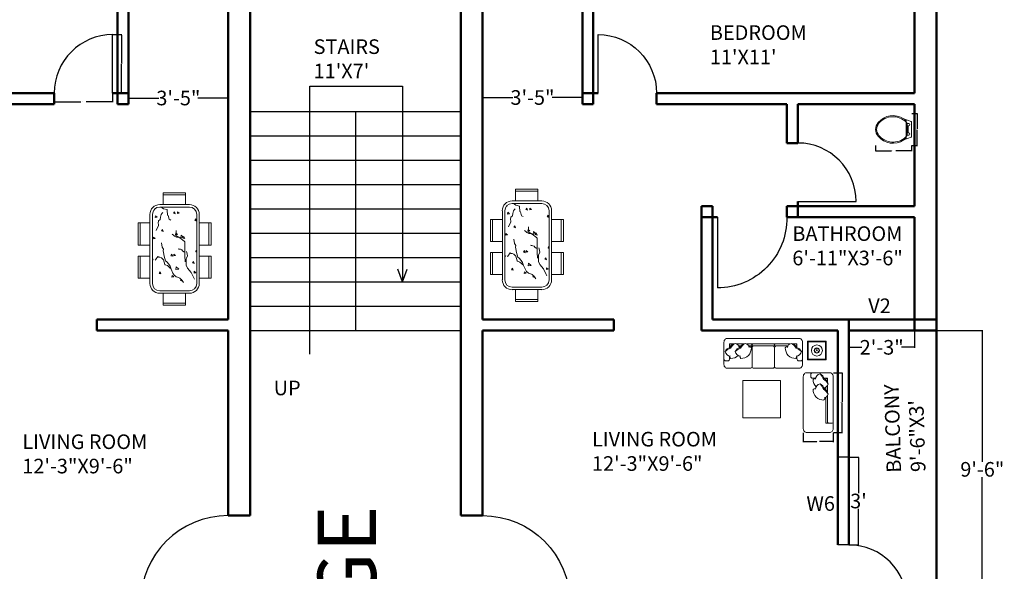
# Model space of a CAD drawing. Units: inches. Extents: x -173 to 545, y -746 to 104.
# Tile 23 of 32: x 125 to 530, y -321 to -94. Entities that reach past the tile are written whole.
import ezdxf

# ---------------------------------------------------------------- set-up
doc = ezdxf.new("R2010")
doc.units = ezdxf.units.IN
doc.header["$MEASUREMENT"] = 0
for name, color, linetype, lineweight in [('A-ANNO-DIMS', 2, 'Continuous', 18), ('A-ANNO-TEXT', 7, 'Continuous', 18), ('A-AREA-IDEN', 7, 'Continuous', 18), ('A-DOOR', 4, 'Continuous', 25), ('A-FLOR-FIXT', 8, 'Continuous', 18), ('A-FLOR-STRS', 7, 'Continuous', 25), ('A-FURN', 8, 'Continuous', 18), ('A-GLAZ', 3, 'Continuous', 25), ('A-WALL', 7, 'Continuous', 50)]:
    doc.layers.add(name, color=color, linetype=linetype, lineweight=lineweight)
doc.styles.get("Standard").update_dxf_attribs({"font": 'arial.ttf'})
doc.dimstyles.get("Standard").update_dxf_attribs({"dimtxt": 0.18, "dimasz": 0.18, "dimexe": 0.18, "dimexo": 0.0625, "dimgap": 0.09, "dimtad": 0, "dimtih": 1, "dimtoh": 1, "dimdec": 0, "dimzin": 0, "dimdsep": 46, "dimlunit": 3, "dimtxsty": 'Standard', "dimcen": 0.09, "dimadec": 0, "dimazin": 0, "dimtfac": 1, "dimtdec": 0, "dimtofl": 0, "dimtmove": 0, "dimatfit": 3, "dimfxl": 1, "dimtolj": 1, "dimtzin": 0, "dimarcsym": 0})

# ---------------------------------------------------------------- blocks, each defined once
blk = doc.blocks.new('*D1')
at = {"layer": 'A-ANNO-DIMS', "color": 0, "lineweight": -2, "transparency": 16777216}
for p, q in [((169.8, -128.8), (169.8, -126.2)), ((169.98, -126.38), (182.24, -126.38)), ((210.62, -126.38), (198.36, -126.38)), ((210.8, -128.8), (210.8, -126.2))]:
    blk.add_line(p, q, dxfattribs=at)
at = {"layer": 'A-ANNO-DIMS', "color": 0, "transparency": 16777216}
for points in [[(169.98, -126.35), (169.98, -126.41), (169.8, -126.38)], [(210.62, -126.35), (210.62, -126.41), (210.8, -126.38)]]:
    blk.add_solid(points, dxfattribs=at)
at = {"layer": 'Defpoints', "color": 0, "transparency": 16777216}
for p in [(169.8, -128.86), (210.8, -126.38), (210.8, -128.86)]:
    blk.add_point(p, dxfattribs=at)
at = {"layer": 'A-ANNO-DIMS', "color": 0, "transparency": 16777216, "insert": (190.3, -126.38), "char_height": 6, "attachment_point": 5}
blk.add_mtext('\\A1;3\'-5"', dxfattribs=at)
blk = doc.blocks.new('*D4')
at = {"layer": 'A-ANNO-DIMS', "color": 0, "lineweight": -2, "transparency": 16777216}
for p, q in [((315.3, -128.8), (315.3, -125.99)), ((315.48, -126.17), (327.74, -126.17)), ((356.12, -126.17), (343.86, -126.17)), ((356.3, -128.8), (356.3, -125.99))]:
    blk.add_line(p, q, dxfattribs=at)
at = {"layer": 'A-ANNO-DIMS', "color": 0, "transparency": 16777216}
for points in [[(315.48, -126.14), (315.48, -126.2), (315.3, -126.17)], [(356.12, -126.14), (356.12, -126.2), (356.3, -126.17)]]:
    blk.add_solid(points, dxfattribs=at)
at = {"layer": 'Defpoints', "color": 0, "transparency": 16777216}
for p in [(315.3, -126.17), (315.3, -128.86), (356.3, -128.86)]:
    blk.add_point(p, dxfattribs=at)
at = {"layer": 'A-ANNO-DIMS', "color": 0, "transparency": 16777216, "insert": (335.8, -126.17), "char_height": 6, "attachment_point": 5}
blk.add_mtext('\\A1;3\'-5"', dxfattribs=at)
blk = doc.blocks.new('*D5')
at = {"layer": 'A-ANNO-DIMS', "color": 0, "lineweight": -2, "transparency": 16777216}
for p, q in [((465.8, -221.92), (465.8, -228.94)), ((492.8, -221.92), (492.8, -228.94)), ((465.98, -228.76), (471.19, -228.76)), ((492.62, -228.76), (487.42, -228.76))]:
    blk.add_line(p, q, dxfattribs=at)
at = {"layer": 'A-ANNO-DIMS', "color": 0, "transparency": 16777216}
for points in [[(465.98, -228.73), (465.98, -228.79), (465.8, -228.76)], [(492.62, -228.73), (492.62, -228.79), (492.8, -228.76)]]:
    blk.add_solid(points, dxfattribs=at)
at = {"layer": 'Defpoints', "color": 0, "transparency": 16777216}
for p in [(465.8, -221.86), (492.8, -221.86), (492.8, -228.76)]:
    blk.add_point(p, dxfattribs=at)
at = {"layer": 'A-ANNO-DIMS', "color": 0, "transparency": 16777216, "insert": (479.3, -228.76), "char_height": 6, "attachment_point": 5}
blk.add_mtext('\\A1;2\'-3"', dxfattribs=at)
blk = doc.blocks.new('*D6')
at = {"layer": 'A-ANNO-DIMS', "color": 0, "lineweight": -2, "transparency": 16777216}
for p, q in [((465.86, -273.86), (469.93, -273.86)), ((469.75, -274.04), (469.75, -288.71)), ((469.75, -309.68), (469.75, -295.02)), ((465.86, -309.86), (469.93, -309.86))]:
    blk.add_line(p, q, dxfattribs=at)
at = {"layer": 'A-ANNO-DIMS', "color": 0, "transparency": 16777216}
for points in [[(469.72, -274.04), (469.78, -274.04), (469.75, -273.86)], [(469.72, -309.68), (469.78, -309.68), (469.75, -309.86)]]:
    blk.add_solid(points, dxfattribs=at)
at = {"layer": 'Defpoints', "color": 0, "transparency": 16777216}
for p in [(465.8, -273.86), (465.8, -309.86), (469.75, -309.86)]:
    blk.add_point(p, dxfattribs=at)
at = {"layer": 'A-ANNO-DIMS', "color": 0, "transparency": 16777216, "insert": (469.75, -291.86), "char_height": 6, "attachment_point": 5}
blk.add_mtext("\\A1;3'", dxfattribs=at)
blk = doc.blocks.new('*D8')
at = {"layer": 'A-ANNO-DIMS', "color": 0, "lineweight": -2, "transparency": 16777216}
for p, q in [((501.86, -221.86), (520.82, -221.86)), ((520.64, -222.04), (520.64, -275.71)), ((520.64, -335.68), (520.64, -282.02)), ((501.86, -335.86), (520.82, -335.86))]:
    blk.add_line(p, q, dxfattribs=at)
at = {"layer": 'A-ANNO-DIMS', "color": 0, "transparency": 16777216}
for points in [[(520.61, -222.04), (520.67, -222.04), (520.64, -221.86)], [(520.61, -335.68), (520.67, -335.68), (520.64, -335.86)]]:
    blk.add_solid(points, dxfattribs=at)
at = {"layer": 'Defpoints', "color": 0, "transparency": 16777216}
for p in [(501.8, -221.86), (501.8, -335.86), (520.64, -335.86)]:
    blk.add_point(p, dxfattribs=at)
at = {"layer": 'A-ANNO-DIMS', "color": 0, "transparency": 16777216, "insert": (520.64, -278.86), "char_height": 6, "attachment_point": 5}
blk.add_mtext('\\A1;9\'-6"', dxfattribs=at)
blk = doc.blocks.new('DAY BED1')
at = {"color": 0}
blk.add_line((0.3, 0.25), (0.225, 0.255), dxfattribs=at)
blk.add_lwpolyline([(-0.3, 0, -0.414214), (-0.4, 0.1), (-0.4, 0.1, 0.317837), (-0.4, 0.1, -0.414214), (-0.4, 0.1), (-0.4, 0.1, 1.186185), (-0.4, 0.1, -0.414214), (-0.4, 0.1), (-0.4, 1.5, -0.414214), (-0.3, 1.6), (0.3, 1.6, -0.414214), (0.4, 1.5), (0.4, 0.1, -0.414214), (0.3, 0)], format="xyb", close=True, dxfattribs=at)
for points in [[(-0.073, 1.45), (-0.15, 1.45, -0.414214), (-0.2, 1.5), (-0.2, 1.55, -0.414214), (-0.15, 1.6)], [(-0.073, 1.45, 0.165541), (-0.139, 1.419, 0.200231), (-0.058, 1.221, 0.121523)], [(-0.076, 1.425, -0.356772), (0.05, 1.568, -0.249542), (0.154, 1.438, 9.61688)], [(0.05, 1.568, -0.14773), (0.136, 1.422, -0.213343), (0.262, 1.293, -0.178662)], [(0.143, 1.442, -0.306663), (0.262, 1.293, -0.30633), (0.154, 1.196, 0.872847)], [(0.25, 1.345), (0.25, 1.45), (0.152, 1.45, -0.414214)], [(0.2, 1.412), (0.2, 1.43, -0.414214), (0.22, 1.45), (0.23, 1.45, -0.414214), (0.25, 1.43)], [(0.25, 1.43), (0.25, 1.345, -0.414214)], [(-0.073, 1.181, 0.165541), (-0.139, 1.15, 0.425989), (0.148, 0.869, 0.121523), (0.187, 0.936, -7.115464)], [(-0.076, 1.156, -0.356772), (0.05, 1.299, -0.249542), (0.154, 1.169, 9.61688)], [(0.05, 1.299, -0.14773), (0.136, 1.153, -0.213343), (0.262, 1.024, -0.178662)], [(0.143, 1.173, -0.306663), (0.262, 1.024, -0.30633), (0.154, 0.926, 0.872847)], [(0.168, 1.163, 0.071865), (0.187, 1.205, -7.115464)], [(0.2, 1.142), (0.2, 1.211, -0.414214)], [(0.25, 1.262), (0.25, 1.075, -0.414214)], [(0.25, 0.992), (0.25, 0.275, -0.414214), (0.23, 0.255), (0.22, 0.255, -0.414214), (0.2, 0.275), (0.2, 0.942, -0.414214)], [(0.25, 0.377), (0.25, 0.3, 0.414214), (0.3, 0.25), (0.35, 0.25, 0.414214), (0.4, 0.3)]]:
    blk.add_lwpolyline(points, format="xyb", dxfattribs=at)
for points in [[(0.25, 1.075), (0.25, 1.262)], [(0.25, 0.377), (0.25, 0.992)]]:
    blk.add_lwpolyline(points, dxfattribs=at)
blk = doc.blocks.new('DINING-TABLE-SIX')
for p, q in [((19.42, 46.17), (10.32, 46.17)), ((10.32, 46.17), (10.32, 41.3)), ((10.32, 45.28), (19.42, 45.28)), ((19.42, 41.3), (19.42, 46.17)), ((21.06, 41.3), (8.92, 41.3)), ((4.88, 37.25), (4.88, 8.92)), ((5.89, 8.92), (5.89, 37.25)), ((6.49, 39.07), (6.86, 39.11)), ((6.68, 39.29), (6.86, 39.11)), ((7.08, 36.66), (7.02, 35.94)), ((7.08, 36.66), (7.78, 36.08)), ((8.92, 40.29), (21.06, 40.29)), ((9.17, 36.14), (9.5, 37.24)), ((9.38, 40.21), (9.93, 39.99)), ((9.5, 37.24), (9.94, 37.79)), ((9.93, 39.99), (10.48, 39.55)), ((9.94, 37.79), (10.16, 38.12)), ((10.48, 39.55), (11.91, 39.22)), ((11.91, 39.22), (11.91, 39)), ((11.91, 39), (12.13, 37.02)), ((12.13, 37.02), (12.35, 36.8)), ((12.35, 36.8), (12.79, 35.26)), ((14.89, 38.37), (14.48, 37.76)), ((14.48, 37.76), (15.22, 37.52)), ((14.89, 38.37), (15.22, 37.52)), ((16.21, 38.35), (16.15, 37.62)), ((16.15, 37.62), (16.91, 37.76)), ((16.21, 38.35), (16.91, 37.76)), ((24.1, 37.25), (24.1, 8.92)), ((25.11, 8.92), (25.11, 37.25)), ((4.88, 33.75), (0, 33.75)), ((0, 33.75), (0, 24.64)), ((0.89, 24.64), (0.89, 33.75)), ((7.02, 35.94), (7.78, 36.08)), ((7.41, 30.64), (8.4, 32.73)), ((8.18, 33.72), (8.4, 34.6)), ((8.4, 33.17), (8.18, 33.72)), ((8.4, 34.6), (9.06, 35.15)), ((8.4, 32.73), (8.4, 33.17)), ((9.06, 35.15), (9.17, 36.14)), ((12.79, 35.26), (13.45, 34.93)), ((23.69, 35.41), (23.29, 34.81)), ((23.29, 34.81), (24.02, 34.56)), ((23.69, 35.41), (24.02, 34.56)), ((25.11, 33.75), (29.99, 33.75)), ((29.1, 24.64), (29.1, 33.75)), ((29.99, 33.75), (29.99, 24.64)), ((9.59, 30.52), (10.33, 30.27)), ((10, 31.12), (9.6, 30.52)), ((10, 31.12), (10.33, 30.27)), ((14.55, 28.77), (14, 29.21)), ((14.99, 28.33), (14.55, 28.77)), ((15.76, 27.89), (14.99, 28.33)), ((15.45, 29.64), (15.39, 28.91)), ((15.39, 28.91), (16.15, 29.05)), ((15.43, 28.66), (15.65, 30.31)), ((17.08, 27.67), (15.43, 28.66)), ((15.45, 29.64), (16.15, 29.05)), ((15.65, 30.31), (15.65, 30.64)), ((17.7, 28.71), (17.54, 27.63)), ((17.7, 28.71), (18.69, 27.77)), ((0, 24.64), (4.88, 24.64)), ((6.32, 27.95), (6.25, 27.23)), ((6.25, 27.23), (7.02, 27.37)), ((6.32, 27.95), (7.02, 27.37)), ((9.93, 23.82), (9.6, 25.58)), ((16.75, 27.89), (15.76, 27.89)), ((18.94, 26.24), (17.08, 27.67)), ((17.54, 27.63), (18.69, 27.77)), ((18.81, 28.17), (18.4, 27.56)), ((18.4, 27.56), (19.13, 27.32)), ((18.81, 28.17), (19.13, 27.32)), ((19.16, 26.02), (18.94, 26.24)), ((19.16, 19.64), (19.16, 26.02)), ((29.99, 24.64), (25.11, 24.64)), ((10.48, 23.05), (9.93, 23.82)), ((10.26, 22.28), (10.48, 23.05)), ((10.48, 21.62), (10.26, 22.28)), ((10.7, 20.19), (10.48, 21.62)), ((13.92, 20.92), (13.51, 20.32)), ((13.51, 20.32), (14.24, 20.07)), ((13.92, 20.92), (14.24, 20.07)), ((14.69, 20.93), (14.62, 20.21)), ((14.62, 20.21), (15.39, 20.35)), ((14.69, 20.93), (15.39, 20.35)), ((16.75, 23.05), (16.42, 23.16)), ((16.97, 23.05), (16.75, 23.05)), ((17.41, 22.94), (16.97, 23.05)), ((17.96, 22.72), (17.41, 22.94)), ((18.29, 22.28), (17.96, 22.72)), ((18.84, 21.95), (18.29, 22.28)), ((19.17, 21.73), (18.84, 21.95)), ((19.71, 18.98), (20.26, 20.3)), ((20.04, 21.62), (19.93, 22.06)), ((20.26, 20.3), (20.04, 21.62)), ((23.82, 22.62), (23.76, 21.89)), ((23.76, 21.89), (24.1, 21.95)), ((23.82, 22.62), (24.1, 22.38)), ((4.88, 20.19), (0, 20.19)), ((0, 20.19), (0, 11.09)), ((0.89, 11.09), (0.89, 20.19)), ((5.89, 18.97), (6.25, 18.66)), ((5.89, 18.59), (6.25, 18.66)), ((7.19, 18.65), (6.97, 18.43)), ((8.07, 19.97), (7.19, 18.65)), ((8.51, 19.75), (8.07, 19.97)), ((8.94, 19.75), (8.51, 19.75)), ((9.6, 19.42), (8.94, 19.75)), ((10.37, 18.65), (9.6, 19.42)), ((10.92, 16.67), (10.37, 18.65)), ((11.25, 18.21), (10.7, 20.19)), ((11.14, 16.56), (10.92, 16.67)), ((12.13, 16.23), (11.14, 16.56)), ((11.8, 17.77), (11.25, 18.21)), ((12.57, 16.89), (11.8, 17.77)), ((12.9, 15.46), (12.13, 16.23)), ((13.23, 16.01), (12.57, 16.89)), ((19.38, 18.43), (19.16, 19.64)), ((19.38, 17.77), (19.38, 18.43)), ((19.71, 16.45), (19.71, 18.98)), ((20.26, 15.24), (19.71, 16.45)), ((22.72, 17.97), (22.31, 17.36)), ((22.31, 17.36), (23.05, 17.12)), ((22.72, 17.97), (23.05, 17.12)), ((25.11, 20.19), (29.99, 20.19)), ((29.1, 11.09), (29.1, 20.19)), ((29.99, 20.19), (29.99, 11.09)), ((9.03, 13.67), (8.62, 13.07)), ((8.62, 13.07), (9.36, 12.82)), ((9.03, 13.67), (9.36, 12.82)), ((13.34, 15.02), (12.9, 15.46)), ((13.56, 14.8), (13.23, 16.01)), ((14.33, 13.15), (13.56, 14.8)), ((13.93, 12.22), (13.86, 11.5)), ((13.93, 12.22), (14.62, 11.64)), ((14.77, 12.38), (14.33, 13.15)), ((15.32, 11.94), (14.77, 12.38)), ((15.69, 15.75), (15.53, 14.68)), ((15.53, 14.68), (16.68, 14.81)), ((15.69, 15.75), (16.68, 14.81)), ((21.8, 13.37), (20.26, 15.24)), ((22.9, 11.17), (21.8, 13.37)), ((23.06, 13.91), (22.99, 13.18)), ((22.99, 13.18), (23.76, 13.32)), ((23.06, 13.91), (23.76, 13.32)), ((0, 11.09), (4.88, 11.09)), ((13.86, 11.5), (14.62, 11.64)), ((15.65, 11.61), (15.32, 11.94)), ((16.2, 11.5), (15.65, 11.61)), ((17.19, 11.06), (16.2, 11.5)), ((18.07, 10.18), (17.19, 11.06)), ((17.83, 10.72), (17.43, 10.11)), ((17.43, 10.11), (18.16, 9.87)), ((17.83, 10.72), (18.16, 9.87)), ((18.61, 9.3), (18.07, 10.18)), ((23.12, 10.62), (22.9, 11.17)), ((29.99, 11.09), (25.11, 11.09)), ((21.06, 5.89), (8.92, 5.89)), ((8.92, 4.88), (21.06, 4.88)), ((10.32, 4.88), (10.32, 0)), ((19.42, 0), (19.42, 4.88)), ((19.42, 0.89), (10.32, 0.89)), ((10.32, 0), (19.42, 0))]:
    blk.add_line(p, q)
for centre, radius, start, end in [((8.92, 37.25), 4.05, 90, 180), ((21.06, 37.25), 4.05, 0, 90), ((8.92, 37.25), 3.04, 90, 180), ((21.06, 37.25), 3.04, 0, 90), ((8.92, 8.92), 4.05, 180, 270), ((8.92, 8.92), 3.04, 180, 270), ((21.06, 8.92), 3.04, 270, 0), ((21.06, 8.92), 4.05, 270, 0)]:
    blk.add_arc(centre, radius, start, end)
blk = doc.blocks.new('WC-STANDARD')
for p, q in [((12.59, 8.59), (12.59, 9.21)), ((12.59, 8.59), (12.59, 5.67)), ((12.59, 2.75), (12.59, 5.67)), ((12.59, 2.13), (12.59, 2.75))]:
    blk.add_line(p, q)
for points in [[(11.57, 10.01, 0.383919), (1.07, 8.46, 0.163732), (0, 5.67, 0.359733)], [(12.59, 8.59, 0.448546), (1.41, 8.18, 0.162618), (0.44, 5.67, 0.470877)], [(12.59, 9.21, 0.040937), (11.57, 10.01, 0.163732)], [(14.84, 5.67), (14.84, 8.5, 0.31031), (14.6, 8.85), (11.57, 10.01, 0.209071)], [(13.04, 8.08, 0.022712), (12.59, 8.59, 0.162618)], [(11.57, 1.32, -0.383919), (1.07, 2.88, -0.163732), (0, 5.67, -0.359733)], [(12.29, 2.45, -0.431639), (1.41, 3.16, -0.162618), (0.44, 5.67, -0.470877)], [(14.84, 5.67), (14.84, 2.84, -0.31031), (14.6, 2.49), (11.57, 1.32, -0.209071)], [(13.04, 5.67), (13.04, 8.08, 0.476108)], [(13.04, 8.08), (13.66, 8.08, -1), (13.66, 7.13), (13.34, 7.13)], [(13.04, 5.67), (13.04, 3.26, -0.022712)], [(13.04, 3.26), (13.66, 3.26, 1), (13.66, 4.21), (13.34, 4.21)], [(12.59, 2.13, -0.040937), (11.57, 1.32, -0.163732)], [(12.59, 2.75, -0.014165), (12.29, 2.45, -0.162618)], [(13.04, 3.26, -0.022712), (12.59, 2.75, -0.162618)]]:
    blk.add_lwpolyline(points, format="xyb")
for points in [[(13.34, 7.13), (13.04, 7.13)], [(13.34, 4.21), (13.04, 4.21)], [(13.34, 7.13), (13.34, 4.21)]]:
    blk.add_lwpolyline(points)
blk = doc.blocks.new('DOOR-24')
blk.add_line((24, 0), (24, 24))
blk.add_arc((24, 0), 24, 90, 180)
blk = doc.blocks.new('DOOR-36')
blk.add_line((36, 0), (0, 0))
blk.add_arc((36, 0), 36, 90, 180)
blk = doc.blocks.new('DOOR-BATH-29')
for p, q in [((28.5, 29), (28.5, 5)), ((28.5, 5), (28.5, 0))]:
    blk.add_line(p, q)
blk.add_arc((28.5, 28.5), 28.5, 179.0036, 270)
blk = doc.blocks.new('*D40')
at = {"layer": 'A-ANNO-DIMS', "color": 0, "lineweight": -2, "transparency": 16777216}
for p, q in [((139.3, -124.42), (139.3, -128.14)), ((163.3, -124.42), (163.3, -128.14)), ((139.48, -127.96), (150.26, -127.96)), ((163.12, -127.96), (152.35, -127.96))]:
    blk.add_line(p, q, dxfattribs=at)
at = {"layer": 'A-ANNO-DIMS', "color": 0, "transparency": 16777216}
for points in [[(139.48, -127.93), (139.48, -127.99), (139.3, -127.96)], [(163.12, -127.93), (163.12, -127.99), (163.3, -127.96)]]:
    blk.add_solid(points, dxfattribs=at)
at = {"layer": 'Defpoints', "color": 0, "transparency": 16777216}
for p in [(139.3, -124.36), (163.3, -124.36), (163.3, -127.96)]:
    blk.add_point(p, dxfattribs=at)
at = {"layer": 'A-ANNO-DIMS', "color": 0, "transparency": 16777216, "insert": (151.3, -127.96), "char_height": 0.18, "attachment_point": 5}
blk.add_mtext('\\A1;DOOR 2\'-0" TYP.', dxfattribs=at)
blk = doc.blocks.new('*D41')
at = {"layer": 'A-ANNO-DIMS', "color": 0, "lineweight": -2, "transparency": 16777216}
for p, q in [((163.36, -100.36), (167.08, -100.36)), ((166.9, -100.54), (166.9, -112.18)), ((166.9, -124.18), (166.9, -112.54)), ((163.36, -124.36), (167.08, -124.36))]:
    blk.add_line(p, q, dxfattribs=at)
at = {"layer": 'A-ANNO-DIMS', "color": 0, "transparency": 16777216}
for points in [[(166.87, -100.54), (166.93, -100.54), (166.9, -100.36)], [(166.87, -124.18), (166.93, -124.18), (166.9, -124.36)]]:
    blk.add_solid(points, dxfattribs=at)
at = {"layer": 'Defpoints', "color": 0, "transparency": 16777216}
for p in [(163.3, -100.36), (166.9, -100.36), (163.3, -124.36)]:
    blk.add_point(p, dxfattribs=at)
at = {"layer": 'A-ANNO-DIMS', "color": 0, "transparency": 16777216, "insert": (166.9, -112.36), "char_height": 0.18, "attachment_point": 5}
blk.add_mtext('\\A1;2\'-0" TYP.', dxfattribs=at)
blk = doc.blocks.new('*D46')
at = {"layer": 'A-ANNO-DIMS', "color": 0, "lineweight": -2, "transparency": 16777216}
for p, q in [((459.45, -239.17), (463.26, -239.17)), ((463.08, -239.35), (463.08, -251.3)), ((463.08, -263.6), (463.08, -251.66)), ((459.45, -263.78), (463.26, -263.78))]:
    blk.add_line(p, q, dxfattribs=at)
at = {"layer": 'A-ANNO-DIMS', "color": 0, "transparency": 16777216}
for points in [[(463.05, -239.35), (463.11, -239.35), (463.08, -239.17)], [(463.05, -263.6), (463.11, -263.6), (463.08, -263.78)]]:
    blk.add_solid(points, dxfattribs=at)
at = {"layer": 'Defpoints', "color": 0, "transparency": 16777216}
for p in [(459.39, -239.17), (463.08, -239.17), (459.39, -263.78)]:
    blk.add_point(p, dxfattribs=at)
at = {"layer": 'A-ANNO-DIMS', "color": 0, "transparency": 16777216, "insert": (463.08, -251.48), "char_height": 0.18, "attachment_point": 5}
blk.add_mtext('\\A1;DAY BED 2\'-0 1/2"', dxfattribs=at)
blk = doc.blocks.new('*D47')
at = {"layer": 'A-ANNO-DIMS', "color": 0, "lineweight": -2, "transparency": 16777216}
for p, q in [((447.08, -263.85), (447.08, -267.65)), ((459.39, -263.85), (459.39, -267.65)), ((447.26, -267.47), (452.7, -267.47)), ((459.21, -267.47), (453.77, -267.47))]:
    blk.add_line(p, q, dxfattribs=at)
at = {"layer": 'A-ANNO-DIMS', "color": 0, "transparency": 16777216}
for points in [[(447.26, -267.44), (447.26, -267.5), (447.08, -267.47)], [(459.21, -267.44), (459.21, -267.5), (459.39, -267.47)]]:
    blk.add_solid(points, dxfattribs=at)
at = {"layer": 'Defpoints', "color": 0, "transparency": 16777216}
for p in [(447.08, -263.78), (459.39, -263.78), (459.39, -267.47)]:
    blk.add_point(p, dxfattribs=at)
at = {"layer": 'A-ANNO-DIMS', "color": 0, "transparency": 16777216, "insert": (453.24, -267.47), "char_height": 0.18, "attachment_point": 5}
blk.add_mtext('\\A1;1\'-0 1/2"', dxfattribs=at)
blk = doc.blocks.new('*D66')
at = {"layer": 'A-ANNO-DIMS', "color": 0, "lineweight": -2, "transparency": 16777216}
for p, q in [((476.77, -145.92), (476.77, -148.26)), ((476.95, -148.08), (483.3, -148.08)), ((491.43, -148.08), (485.08, -148.08)), ((491.61, -145.92), (491.61, -148.26))]:
    blk.add_line(p, q, dxfattribs=at)
at = {"layer": 'A-ANNO-DIMS', "color": 0, "transparency": 16777216}
for points in [[(476.95, -148.05), (476.95, -148.11), (476.77, -148.08)], [(491.43, -148.05), (491.43, -148.11), (491.61, -148.08)]]:
    blk.add_solid(points, dxfattribs=at)
at = {"layer": 'Defpoints', "color": 0, "transparency": 16777216}
for p in [(476.77, -145.86), (491.61, -145.86), (491.61, -148.08)]:
    blk.add_point(p, dxfattribs=at)
at = {"layer": 'A-ANNO-DIMS', "color": 0, "transparency": 16777216, "insert": (484.19, -148.08), "char_height": 0.18, "attachment_point": 5}
blk.add_mtext('\\A1;WC 1\'-3" TYP.', dxfattribs=at)
blk = doc.blocks.new('*D67')
at = {"layer": 'A-ANNO-DIMS', "color": 0, "lineweight": -2, "transparency": 16777216}
for p, q in [((491.67, -132.68), (494.01, -132.68)), ((493.83, -132.86), (493.83, -139.09)), ((493.83, -145.68), (493.83, -139.45)), ((491.67, -145.86), (494.01, -145.86))]:
    blk.add_line(p, q, dxfattribs=at)
at = {"layer": 'A-ANNO-DIMS', "color": 0, "transparency": 16777216}
for points in [[(493.8, -132.86), (493.86, -132.86), (493.83, -132.68)], [(493.8, -145.68), (493.86, -145.68), (493.83, -145.86)]]:
    blk.add_solid(points, dxfattribs=at)
at = {"layer": 'Defpoints', "color": 0, "transparency": 16777216}
for p in [(491.61, -132.68), (493.83, -132.68), (491.61, -145.86)]:
    blk.add_point(p, dxfattribs=at)
at = {"layer": 'A-ANNO-DIMS', "color": 0, "transparency": 16777216, "insert": (493.83, -139.27), "char_height": 0.18, "attachment_point": 5}
blk.add_mtext('\\A1;1\'-1" TYP.', dxfattribs=at)

msp = doc.modelspace()

# ---------------------------------------------------------------- linework, layer by layer
at = {"layer": 'A-FLOR-STRS'}
for p, q in [((244.31, -231.63), (244.31, -121.55)), ((244.31, -121.55), (282.43, -121.55)), ((282.43, -121.55), (282.43, -201.86)), ((219.8, -131.86), (306.3, -131.86)), ((263.05, -131.86), (263.05, -221.86)), ((219.8, -141.86), (306.3, -141.86)), ((219.8, -151.86), (306.3, -151.86)), ((219.8, -161.86), (306.3, -161.86)), ((219.8, -171.86), (306.3, -171.86)), ((219.8, -181.86), (306.3, -181.86)), ((219.8, -191.86), (306.3, -191.86)), ((282.43, -201.86), (280.51, -196.65)), ((282.43, -201.86), (284.35, -196.65)), ((219.8, -201.86), (306.3, -201.86)), ((219.8, -211.86), (306.3, -211.86)), ((219.8, -221.86), (306.3, -221.86))]:
    msp.add_line(p, q, dxfattribs=at)
at = {"layer": 'A-FURN'}
for p, q in [((452.63, -230.01), (451.69, -230.55)), ((452.68, -230.09), (451.74, -230.63)), ((452.61, -230.05), (452.61, -228.96)), ((452.63, -230.09), (453.57, -230.63)), ((452.68, -230.01), (453.62, -230.55)), ((452.71, -230.05), (452.71, -228.96))]:
    msp.add_line(p, q, dxfattribs=at)
at = {"layer": 'A-FURN', "ltscale": 0.03}
msp.add_lwpolyline([(446.79, -235.84, -0.414214), (445.25, -237.38), (436.03, -237.38, -0.414214), (435.26, -236.61, -0.414214), (434.49, -237.38), (426.8, -237.38, -0.414214), (426.03, -236.61, -0.414214), (425.26, -237.38), (416.03, -237.38, -0.414214), (414.49, -235.84), (414.49, -226.61, -0.414214), (416.03, -225.07), (445.25, -225.07, -0.414214), (446.79, -226.61)], format="xyb", close=True, dxfattribs=at)
for points in [[(456.5, -233.89), (448.81, -233.89), (448.81, -226.2), (456.5, -226.2)], [(422.28, -257.73), (437.66, -257.73), (437.66, -242.35), (422.28, -242.35)]]:
    msp.add_lwpolyline(points, close=True, dxfattribs=at)
at = {"layer": 'A-FURN'}
msp.add_lwpolyline([(449.12, -233.59), (456.19, -233.59), (456.19, -226.51), (449.12, -226.51)], close=True, dxfattribs=at)
for points in [[(414.98, -230.45, -0.14773), (417.23, -229.13, -0.213343), (419.21, -227.19, -0.178662)], [(417.19, -232.39, -0.356772), (414.98, -230.45, -0.249542), (416.98, -228.85, 9.61688)], [(418.42, -227.38), (416.8, -227.38), (416.8, -228.89, -0.414214)], [(417.39, -228.15), (417.11, -228.15, -0.414214), (416.8, -227.84), (416.8, -227.69, -0.414214), (417.11, -227.38)], [(416.92, -229.02, -0.306663), (419.21, -227.19, -0.30633), (420.71, -228.86, 0.872847)], [(417.11, -227.38), (418.42, -227.38, -0.414214)], [(419.12, -230.45, -0.14773), (421.37, -229.13, -0.213343), (423.36, -227.19, -0.178662)], [(421.33, -232.39, -0.356772), (419.12, -230.45, -0.249542), (421.12, -228.85, 9.61688)], [(419.7, -227.38), (422.56, -227.38, -0.414214)], [(421.53, -228.15), (420.47, -228.15, -0.414214)], [(421.21, -228.64, 0.071865), (420.57, -228.34, -7.115464)], [(420.94, -232.34, 0.165541), (421.42, -233.35, 0.425989), (425.74, -228.95, 0.121523), (424.71, -228.34, -7.115464)], [(421.06, -229.02, -0.306663), (423.36, -227.19, -0.30633), (424.85, -228.86, 0.872847)], [(423.84, -227.38), (425.72, -227.38, -0.414214), (426.03, -227.69), (426.03, -227.84, -0.414214), (425.72, -228.15), (424.61, -228.15, -0.414214)], [(425.26, -228.15, -0.414214), (426.03, -228.92), (426.03, -236.61, -0.414214)], [(426.8, -228.15, 0.414214), (426.03, -228.92)], [(434.49, -228.15, -0.414214), (435.26, -228.92)], [(441.59, -227.38), (435.56, -227.38, 0.414214), (435.26, -227.69), (435.26, -227.84, 0.414214), (435.56, -228.15), (440.81, -228.15, 0.414214)], [(436.03, -228.15, 0.414214), (435.26, -228.92), (435.26, -236.61, 0.414214)], [(444.49, -232.34, -0.165541), (444.01, -233.35, -0.425989), (439.69, -228.95, -0.121523), (440.72, -228.34, 7.115464)], [(444.36, -229.02, 0.306663), (442.07, -227.19, 0.30633), (440.57, -228.86, -0.872847)], [(446.3, -230.45, 0.14773), (444.05, -229.13, 0.213343), (442.07, -227.19, 0.178662)], [(444.18, -227.38), (442.87, -227.38, 0.414214)], [(443.9, -228.15), (444.18, -228.15, 0.414214), (444.48, -227.84), (444.48, -227.69, 0.414214), (444.18, -227.38)], [(444.1, -232.39, 0.356772), (446.3, -230.45, 0.249542), (444.31, -228.85, -9.61688)], [(416.8, -232.34), (416.8, -233.53, -0.414214), (416.03, -234.3), (415.26, -234.3, -0.414214), (414.49, -233.53)], [(416.8, -232.34, 0.165541), (417.27, -233.35, 0.200231), (420.33, -232.12, 0.121523)], [(446.79, -233.53, -0.414214), (446.02, -234.3), (445.25, -234.3, -0.414214), (444.48, -233.53), (444.48, -232.34)]]:
    msp.add_lwpolyline(points, format="xyb", dxfattribs=at)
for points in [[(422.56, -227.38), (419.7, -227.38)], [(441.59, -227.38), (423.84, -227.38)], [(444.48, -228.89), (444.48, -227.38), (442.87, -227.38)]]:
    msp.add_lwpolyline(points, dxfattribs=at)
msp.add_lwpolyline([(426.34, -227.38), (434.95, -227.38, -0.414214), (435.26, -227.69), (435.26, -227.84, -0.414214), (434.95, -228.15), (426.34, -228.15, -0.414214), (426.03, -227.84), (426.03, -227.69, -0.414214)], format="xyb", close=True, dxfattribs=at)
for radius in [2.27, 1.09, 0.973]:
    msp.add_circle((452.66, -230.05), radius, dxfattribs=at)
at = {"layer": 'A-GLAZ'}
for p, q in [((465.8, -273.86), (461.3, -273.86)), ((465.8, -309.86), (461.3, -309.86))]:
    msp.add_line(p, q, dxfattribs=at)
at = {"layer": 'A-WALL'}
for p, q in [((165.3, 7.64), (165.3, -128.86)), ((169.8, 7.64), (169.8, -128.86)), ((356.3, 7.64), (356.3, -128.86)), ((360.8, 7.64), (360.8, -128.86)), ((492.8, 7.64), (492.8, -124.36)), ((501.8, 7.64), (501.8, -697.36)), ((210.8, -81.36), (210.8, -128.86)), ((315.3, -81.36), (315.3, -128.86)), ((219.8, -90.36), (219.8, -128.86)), ((306.3, -90.36), (306.3, -128.86)), ((33.3, -124.36), (139.3, -124.36)), ((139.3, -124.36), (139.3, -128.86)), ((163.3, -124.36), (169.8, -124.36)), ((356.3, -124.36), (362.8, -124.36)), ((386.8, -124.36), (386.8, -128.86)), ((386.8, -124.36), (492.8, -124.36)), ((85.8, -128.86), (139.3, -128.86)), ((165.3, -128.86), (169.8, -128.86)), ((210.8, -128.86), (210.8, -217.36)), ((219.8, -128.86), (219.8, -297.86)), ((306.3, -128.86), (306.3, -297.86)), ((315.3, -128.86), (315.3, -217.36)), ((356.3, -128.86), (360.8, -128.86)), ((386.8, -128.86), (440.3, -128.86)), ((440.3, -128.86), (440.3, -144.86)), ((444.8, -128.86), (444.8, -144.86)), ((444.8, -128.86), (492.8, -128.86)), ((492.8, -128.86), (492.8, -170.86)), ((444.8, -144.86), (440.3, -144.86)), ((444.8, -168.86), (444.8, -175.36)), ((405.3, -170.86), (409.8, -170.86)), ((405.3, -170.86), (405.3, -221.86)), ((409.8, -170.86), (409.8, -217.36)), ((440.3, -170.86), (440.3, -175.36)), ((440.3, -170.86), (492.8, -170.86)), ((405.3, -175.36), (411.8, -175.36)), ((440.3, -175.36), (492.8, -175.36)), ((492.8, -175.36), (492.8, -221.86)), ((156.8, -217.36), (210.8, -217.36)), ((156.8, -217.36), (156.8, -221.86)), ((315.3, -217.36), (369.3, -217.36)), ((369.3, -217.36), (369.3, -221.86)), ((409.8, -217.36), (501.8, -217.36)), ((465.8, -217.36), (465.8, -309.86)), ((156.8, -221.86), (210.8, -221.86)), ((210.8, -221.86), (210.8, -297.86)), ((315.3, -221.86), (369.3, -221.86)), ((315.3, -221.86), (315.3, -297.86)), ((405.3, -221.86), (452.3, -221.86)), ((452.3, -221.86), (456.8, -221.86)), ((456.8, -221.86), (461.3, -221.86)), ((461.3, -221.86), (461.3, -309.86)), ((465.8, -221.86), (501.8, -221.86)), ((210.8, -297.86), (219.8, -297.86)), ((315.3, -297.86), (306.3, -297.86))]:
    msp.add_line(p, q, dxfattribs=at)

# ---------------------------------------------------------------- block references
at = {"layer": 'A-DOOR'}
for name, p in [('DOOR-24', (139.3, -124.36)), ('DOOR-36', (174.8, -333.86))]:
    msp.add_blockref(name, p, dxfattribs=at)
at = {"layer": 'A-DOOR', "extrusion": (0, 0, -1), "zscale": -1}
for name, p in [('DOOR-24', (-386.8, -124.36)), ('DOOR-BATH-29', (-440.3, -204.36)), ('DOOR-36', (-351.3, -333.86))]:
    msp.add_blockref(name, p, dxfattribs=at)
at = {"layer": 'A-DOOR'}
for p, rotation in [((444.8, -144.86), 270.0000000000002), ((465.8, -309.86), 270.0000000000001)]:
    msp.add_blockref('DOOR-24', p, dxfattribs=dict(at, rotation=rotation))
at = {"layer": 'A-FLOR-FIXT'}
msp.add_blockref('WC-STANDARD', (476.77, -144.94), dxfattribs=at)
at = {"layer": 'A-FURN'}
for p in [(173.76, -211.45), (318.54, -209.96)]:
    msp.add_blockref('DINING-TABLE-SIX', p, dxfattribs=at)
at = {"layer": 'A-FURN', "ltscale": 0.03, "xscale": 15.38047337869789, "yscale": 15.38047337869789, "zscale": 15.38047337869789}
msp.add_blockref('DAY BED1', (453.24, -263.78), dxfattribs=at)

# ---------------------------------------------------------------- texts
at = {"layer": 'A-ANNO-TEXT', "char_height": 6, "attachment_point": 1}
for s, insert in [('V2', (473.78, -208.7)), ('UP', (229.46, -242.44)), ('W6', (448.35, -289.9))]:
    msp.add_mtext(s, dxfattribs=dict(at, insert=insert))
at = {"layer": 'A-AREA-IDEN', "char_height": 6, "attachment_point": 1}
for s, insert in [("BEDROOM\\P11'X11'", (408.68, -96.52)), ("STAIRS\\P11'X7'", (245.88, -102.29)), ('BATHROOM\\P6\'-11"X3\'-6"', (442.58, -179.07)), ('LIVING ROOM\\P12\'-3"X9\'-6"', (126.18, -264.52)), ('LIVING ROOM\\P12\'-3"X9\'-6"', (360.26, -263.47))]:
    msp.add_mtext(s, dxfattribs=dict(at, insert=insert))
at = {"layer": 'A-AREA-IDEN', "insert": (448.47, -128.86), "char_height": 6, "attachment_point": 1}
msp.add_mtext_dynamic_manual_height_columns('TOILET\\P4\'X3\'-6"', width=0.000000131, gutter_width=1, heights=[0], dxfattribs=at)
at = {"layer": 'A-AREA-IDEN', "attachment_point": 1}
for s, insert, char_height, rotation in [('BALCONY\\P9\'-6"X3\'', (481.33, -280.35), 6, 91.7171), ('PASSAGE', (247.55, -435.15), 24, 90)]:
    msp.add_mtext(s, dxfattribs=dict(at, insert=insert, char_height=char_height, rotation=rotation))

# ---------------------------------------------------------------- dimensions: what is measured, and where the dimension line sits
at = {"layer": 'A-ANNO-DIMS'}
for base, p1, p2, text, picture, middle in [((166.9, -100.36), (163.3, -124.36), (163.3, -100.36), '<> TYP.', '*D41', (166.9, -112.36)), ((493.83, -132.68), (491.61, -145.86), (491.61, -132.68), '<> TYP.', '*D67', (493.83, -139.27)), ((463.08, -239.17), (459.39, -263.78), (459.39, -239.17), 'DAY BED <>', '*D46', (463.08, -251.48))]:
    dim = msp.add_linear_dim(base=base, p1=p1, p2=p2, angle=90, text=text, dimstyle='Standard', override={"dimdec": 1, "dimlfac": 1, "dimrnd": 0, "dimzin": 1, "dimdsep": 46, "dimlunit": 4, "dimfrac": 2}, dxfattribs=at)
    dim.commit()
    dim.dimension.update_dxf_attribs({"geometry": picture, "text_midpoint": middle})
for base, p1, p2, text, picture, middle in [((163.3, -127.96), (139.3, -124.36), (163.3, -124.36), 'DOOR <> TYP.', '*D40', (151.3, -127.96)), ((491.61, -148.08), (476.77, -145.86), (491.61, -145.86), 'WC <> TYP.', '*D66', (484.19, -148.08))]:
    dim = msp.add_linear_dim(base=base, p1=p1, p2=p2, text=text, dimstyle='Standard', override={"dimdec": 1, "dimlfac": 1, "dimrnd": 0, "dimzin": 1, "dimdsep": 46, "dimlunit": 4, "dimfrac": 2}, dxfattribs=at)
    dim.commit()
    dim.dimension.update_dxf_attribs({"geometry": picture, "text_midpoint": middle})
for base, p1, p2, override, picture, middle in [((210.8, -126.38), (169.8, -128.86), (210.8, -128.86), {"dimtxt": 6, "dimclrd": 0, "dimclre": 0, "dimclrt": 0}, '*D1', (190.3, -126.38)), ((315.3, -126.17), (356.3, -128.86), (315.3, -128.86), {"dimtxt": 6, "dimclrd": 0, "dimclre": 0, "dimclrt": 0}, '*D4', (335.8, -126.17)), ((492.8, -228.76), (465.8, -221.86), (492.8, -221.86), {"dimtxt": 6, "dimclrd": 0, "dimclre": 0, "dimclrt": 0}, '*D5', (479.3, -228.76)), ((459.39, -267.47), (447.08, -263.78), (459.39, -263.78), {"dimdec": 1, "dimlfac": 1, "dimrnd": 0, "dimzin": 1, "dimdsep": 46, "dimlunit": 4, "dimfrac": 2}, '*D47', (453.24, -267.47))]:
    dim = msp.add_linear_dim(base=base, p1=p1, p2=p2, dimstyle='Standard', override=override, dxfattribs=at)
    dim.commit()
    dim.dimension.update_dxf_attribs({"geometry": picture, "text_midpoint": middle})
for base, p1, p2, picture, middle in [((520.64, -335.86), (501.8, -221.86), (501.8, -335.86), '*D8', (520.64, -278.86)), ((469.75, -309.86), (465.8, -273.86), (465.8, -309.86), '*D6', (469.75, -291.86))]:
    dim = msp.add_linear_dim(base=base, p1=p1, p2=p2, angle=90, dimstyle='Standard', override={"dimtxt": 6, "dimclrd": 0, "dimclre": 0, "dimclrt": 0}, dxfattribs=at)
    dim.commit()
    dim.dimension.update_dxf_attribs({"geometry": picture, "text_midpoint": middle})

doc.saveas('drawing.dxf')
